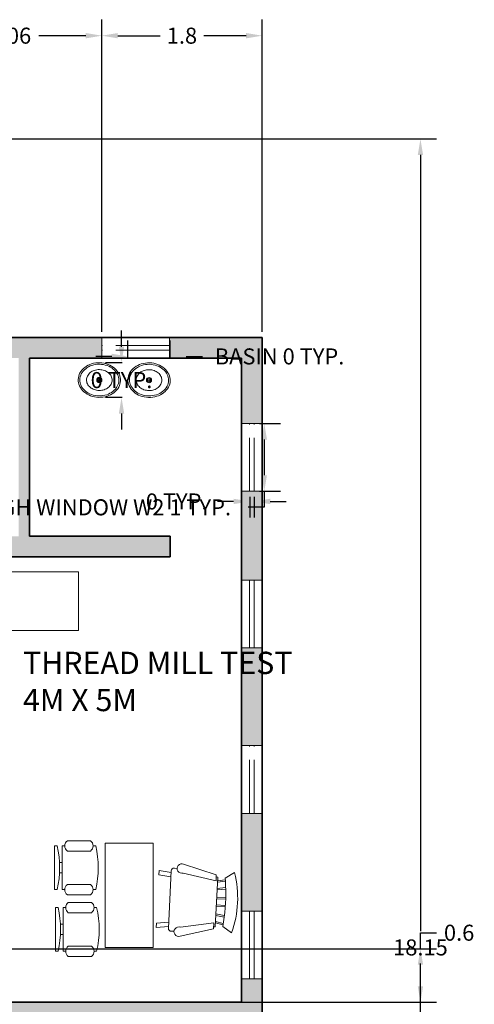
# Model space of a CAD drawing. Units: metres. Extents: x 4298.5 to 4325.2, y 2075 to 2095.8.
# Tile 35 of 35: x 4320.1 to 4325.2, y 2084.8 to 2095.8. Entities that reach past the tile are written whole.
import ezdxf

# ---------------------------------------------------------------- set-up
doc = ezdxf.new("R2010")
doc.units = ezdxf.units.M
doc.linetypes.add('ACAD_ISO02W100', pattern=[15, 12, -3])
for name, color, linetype, lineweight in [('A-ANNO-DIMS', 2, 'Continuous', 18), ('A-AREA-IDEN', 7, 'Continuous', 18), ('A-EQPM', 9, 'Continuous', 18), ('A-FLOR-FIXT', 15, 'Continuous', 18), ('A-FURN', 15, 'Continuous', 18), ('A-GLAZ', 4, 'Continuous', 18), ('A-GLAZ-OVHD', 4, 'ACAD_ISO02W100', 13), ('A-WALL', 7, 'Continuous', 35), ('A-WALL-PATT', 252, 'Continuous', 13)]:
    doc.layers.add(name, color=color, linetype=linetype, lineweight=lineweight)
doc.styles.get("Standard").update_dxf_attribs({"font": 'arial.ttf'})
doc.dimstyles.get("Standard").update_dxf_attribs({"dimtxt": 0.18, "dimasz": 0.18, "dimexe": 0.18, "dimexo": 0.0625, "dimgap": 0.09, "dimtad": 0, "dimtih": 1, "dimtoh": 1, "dimdec": 4, "dimzin": 0, "dimdsep": 46, "dimtxsty": 'Standard', "dimcen": 0.09, "dimadec": 0, "dimazin": 0, "dimtfac": 1, "dimtdec": 4, "dimtofl": 0, "dimtmove": 0, "dimatfit": 3, "dimfxl": 1, "dimtolj": 1, "dimtzin": 0, "dimarcsym": 0})

# ---------------------------------------------------------------- blocks, each defined once
blk = doc.blocks.new('Chair - Desk')
for p, q in [((-8.5, 0), (-8.5, -1)), ((-8.5, 0), (8.5, 0)), ((8.5, 0), (8.5, -1)), ((-8.5, -3), (-8.5, -4)), ((-8.5, -3), (8.5, -3)), ((-2, -3), (-2, -1.9355)), ((2, -1.9576), (2, -3)), ((8.5, -3), (8.5, -4)), ((-10.5, -5), (-10.5, -14)), ((-6.5, -14), (-6.5, -5)), ((6.5, -5), (6.5, -14)), ((10.5, -14), (10.5, -5)), ((-8.5, -15), (-8.5, -16)), ((8.5, -15), (8.5, -16))]:
    blk.add_line(p, q)
for centre, radius, start, end in [((0, 34.625), 36.625, 256.5803, 283.4197), ((-8.5, -6.5), 2.5, 36.8699, 143.1301), ((8.5, -6.5), 2.5, 36.8699, 143.1301), ((-8.5, -12.5), 2.5, 216.8699, 323.1301), ((8.5, -12.5), 2.5, 216.8699, 323.1301), ((0, 19.625), 36.625, 256.5803, 283.4197)]:
    blk.add_arc(centre, radius, start, end)
blk = doc.blocks.new('Chair - Rocking')
for p, q in [((-8, -4.5), (-10, -1.5)), ((8, -4.5), (10, -1.5)), ((-7.5, -4.5), (-7, -7)), ((-6.5, -7), (-7.02225, -4.43)), ((-4.5, -7), (-4.96674, -4.19951)), ((-4, -7), (-4.40532, -4.16272)), ((-1.5, -4.05012), (-1.5, -7)), ((-1, -7), (-1, -4.05012)), ((1, -7), (1, -4.04655)), ((1.5, -4.05012), (1.5, -7)), ((4, -7), (4.40187, -4.18694)), ((4.5, -7), (4.96761, -4.19437)), ((6.5, -7), (7, -4.4057)), ((7.5, -4.5), (7, -7)), ((-9, -7.5), (-12, -18.49999)), ((-7, -7.5), (-9, -7.5)), ((-9, -18.49999), (-7, -7.5)), ((-8.23428, -6.99939), (-8.3093, -7.47958)), ((-8.23041, -7), (8.23915, -7)), ((7, -7.5), (9, -7.5)), ((9, -18.49999), (7, -7.5)), ((8.31071, -7.48854), (8.23449, -7.00073)), ((9, -7.5), (12, -18.49999)), ((-10.36644, -20.64523), (-10.5, -21.49999)), ((-9, -22.49999), (-9.5, -26.49999)), ((0, -22.49999), (-9.5, -22.49999)), ((-8, -26.49999), (-7.5, -22.49999)), ((0, -22.49999), (9.5, -22.49999)), ((8, -26.49999), (7.5, -22.49999)), ((9, -22.49999), (9.5, -26.49999)), ((10.5, -21.49999), (10.3575, -20.58798)), ((-9.5, -26.49999), (-8, -26.49999)), ((9.5, -26.49999), (8, -26.49999))]:
    blk.add_line(p, q)
for centre, radius, start, end in [((0, -34.08333), 34.08333, 72.93847, 107.0615), ((0, -68.25004), 64.25, 93.92211, 97.15267), ((0, -68.25004), 64.25, 82.84733, 93.92211), ((-10.5, -18.99999), 1.58114, 161.5651, 18.43495), ((10.5, -18.99999), 1.58114, 161.5651, 18.43495), ((-9.5, -21.49999), 1, 180, 270), ((9.5, -21.49999), 1, 270, 0)]:
    blk.add_arc(centre, radius, start, end)
blk = doc.blocks.new('Sink - Oval top')
for p, q in [((-1, 0), (1, 0)), ((0, 1), (0, -1))]:
    blk.add_line(p, q)
for points in [[(-12.23, 0.39, 0.117634), (-11.46, -3.36, 0.104469), (-8.88, -6.8, 0.090016), (-5.08, -9.07, 0.08192), (-0.32, -10.02, 0.08192), (4.49, -9.38, 0.090016), (8.42, -7.36, 0.104469), (11.22, -4.09, 0.117634), (12.23, -0.39, 0.117634), (11.46, 3.36, 0.104469), (8.88, 6.8, 0.090016), (5.08, 9.07, 0.08192), (0.32, 10.02, 0.08192), (-4.49, 9.38, 0.090016), (-8.42, 7.36, 0.104469), (-11.22, 4.09, 0.117634)], [(-11.29, 0.16, 0.118622), (-10.52, -3.25, 0.104678), (-8.07, -6.36, 0.089562), (-4.54, -8.37, 0.081185), (-0.13, -9.15, 0.081185), (4.3, -8.49, 0.089562), (7.89, -6.58, 0.104678), (10.42, -3.55, 0.118622), (11.29, -0.16, 0.118622), (10.52, 3.25, 0.104678), (8.07, 6.36, 0.089562), (4.54, 8.37, 0.081185), (0.13, 9.15, 0.081185), (-4.3, 8.49, 0.089562), (-7.89, 6.58, 0.104678), (-10.42, 3.55, 0.118622)], [(-7.42, 0.08, 0.118283), (-6.91, -2.17, 0.104607), (-5.29, -4.21, 0.089718), (-2.97, -5.53, 0.081436), (-0.07, -6.04, 0.081436), (2.84, -5.59, 0.089718), (5.2, -4.33, 0.104607), (6.86, -2.32, 0.118283), (7.42, -0.08, 0.118283), (6.91, 2.17, 0.104607), (5.29, 4.21, 0.089718), (2.97, 5.53, 0.081436), (0.07, 6.04, 0.081436), (-2.84, 5.59, 0.089718), (-5.2, 4.33, 0.104607), (-6.86, 2.32, 0.118283)]]:
    blk.add_lwpolyline(points, format="xyb", close=True)
for radius in [1.5, 1]:
    blk.add_circle((0, 0), radius)
blk = doc.blocks.new('WIN-760-GLASS-HIGH')
at = {"ltscale": 0.05}
for p, q in [((0, 0.76), (0, 0)), ((0.05, 0.76), (0.05, 0))]:
    blk.add_line(p, q, dxfattribs=at)
blk = doc.blocks.new('WIN-760-GLASS')
for p, q in [((0, 0.76), (0, 0)), ((0.05, 0.76), (0.05, 0))]:
    blk.add_line(p, q)
blk = doc.blocks.new('DESK-1175')
blk.add_lwpolyline([(0, 1.173), (0.538, 1.173), (0.538, 0), (0, 0)], close=True)
blk = doc.blocks.new('*D21')
at = {"layer": 'A-ANNO-DIMS', "color": 0, "lineweight": -2, "transparency": 16777216}
for p, q in [((4321.304, 2092.028), (4321.304, 2092.217)), ((4321.78, 2092.028), (4321.78, 2092.217)), ((4321.124, 2092.037), (4320.944, 2092.037)), ((4321.96, 2092.037), (4322.14, 2092.037))]:
    blk.add_line(p, q, dxfattribs=at)
at = {"layer": 'A-ANNO-DIMS', "color": 0, "transparency": 16777216}
for points in [[(4321.124, 2092.067), (4321.124, 2092.007), (4321.304, 2092.037)], [(4321.96, 2092.067), (4321.96, 2092.007), (4321.78, 2092.037)]]:
    blk.add_solid(points, dxfattribs=at)
at = {"layer": 'Defpoints', "color": 0, "transparency": 16777216}
for p in [(4321.304, 2091.966), (4321.78, 2092.037), (4321.78, 2091.966)]:
    blk.add_point(p, dxfattribs=at)
at = {"layer": 'A-ANNO-DIMS', "color": 0, "transparency": 16777216, "insert": (4323.006, 2092.037), "char_height": 0.18, "attachment_point": 5}
blk.add_mtext('\\A1;BASIN 0 TYP.', dxfattribs=at)
blk = doc.blocks.new('*D22')
at = {"layer": 'A-ANNO-DIMS', "color": 0, "lineweight": -2, "transparency": 16777216}
for p, q in [((4321.233, 2092.146), (4321.233, 2092.326)), ((4321.241, 2091.966), (4321.053, 2091.966)), ((4321.241, 2091.576), (4321.053, 2091.576)), ((4321.233, 2091.396), (4321.233, 2091.216))]:
    blk.add_line(p, q, dxfattribs=at)
at = {"layer": 'A-ANNO-DIMS', "color": 0, "transparency": 16777216}
for points in [[(4321.203, 2092.146), (4321.263, 2092.146), (4321.233, 2091.966)], [(4321.203, 2091.396), (4321.263, 2091.396), (4321.233, 2091.576)]]:
    blk.add_solid(points, dxfattribs=at)
at = {"layer": 'Defpoints', "color": 0, "transparency": 16777216}
for p in [(4321.233, 2091.966), (4321.304, 2091.966), (4321.304, 2091.576)]:
    blk.add_point(p, dxfattribs=at)
at = {"layer": 'A-ANNO-DIMS', "color": 0, "transparency": 16777216, "insert": (4321.233, 2091.771), "char_height": 0.18, "attachment_point": 5}
blk.add_mtext('\\A1;0 TYP.', dxfattribs=at)
blk = doc.blocks.new('*D25')
at = {"layer": 'A-ANNO-DIMS', "color": 0, "lineweight": -2, "transparency": 16777216}
for p, q in [((4322.783, 2091.283), (4323.015, 2091.283)), ((4322.835, 2091.103), (4322.835, 2090.703)), ((4322.783, 2090.523), (4323.015, 2090.523)), ((4322.835, 2090.523), (4322.835, 2090.343)), ((4322.835, 2090.343), (4322.655, 2090.343))]:
    blk.add_line(p, q, dxfattribs=at)
at = {"layer": 'A-ANNO-DIMS', "color": 0, "transparency": 16777216}
for points in [[(4322.805, 2091.103), (4322.865, 2091.103), (4322.835, 2091.283)], [(4322.805, 2090.703), (4322.865, 2090.703), (4322.835, 2090.523)]]:
    blk.add_solid(points, dxfattribs=at)
at = {"layer": 'Defpoints', "color": 0, "transparency": 16777216}
for p in [(4322.721, 2091.283), (4322.721, 2090.523), (4322.835, 2090.523)]:
    blk.add_point(p, dxfattribs=at)
at = {"layer": 'A-ANNO-DIMS', "color": 0, "transparency": 16777216, "insert": (4321.042, 2090.343), "char_height": 0.18, "attachment_point": 5}
blk.add_mtext('\\A1;HIGH WINDOW W2 1 TYP.', dxfattribs=at)
blk = doc.blocks.new('*D26')
at = {"layer": 'A-ANNO-DIMS', "color": 0, "lineweight": -2, "transparency": 16777216}
for p, q in [((4322.491, 2090.409), (4322.311, 2090.409)), ((4322.671, 2090.461), (4322.671, 2090.229)), ((4322.721, 2090.461), (4322.721, 2090.229)), ((4322.901, 2090.409), (4323.081, 2090.409))]:
    blk.add_line(p, q, dxfattribs=at)
at = {"layer": 'A-ANNO-DIMS', "color": 0, "transparency": 16777216}
for points in [[(4322.491, 2090.439), (4322.491, 2090.379), (4322.671, 2090.409)], [(4322.901, 2090.439), (4322.901, 2090.379), (4322.721, 2090.409)]]:
    blk.add_solid(points, dxfattribs=at)
at = {"layer": 'Defpoints', "color": 0, "transparency": 16777216}
for p in [(4322.671, 2090.523), (4322.721, 2090.523), (4322.671, 2090.409)]:
    blk.add_point(p, dxfattribs=at)
at = {"layer": 'A-ANNO-DIMS', "color": 0, "transparency": 16777216, "insert": (4321.852, 2090.409), "char_height": 0.18, "attachment_point": 5}
blk.add_mtext('\\A1;0 TYP.', dxfattribs=at)
blk = doc.blocks.new('*D48')
at = {"layer": 'A-ANNO-DIMS', "color": 0, "lineweight": -2, "transparency": 16777216}
for p, q in [((4310.183, 2094.478), (4324.767, 2094.478)), ((4324.587, 2094.298), (4324.587, 2085.585)), ((4324.587, 2076.508), (4324.587, 2085.221)), ((4316.873, 2076.328), (4324.767, 2076.328))]:
    blk.add_line(p, q, dxfattribs=at)
at = {"layer": 'A-ANNO-DIMS', "color": 0, "transparency": 16777216}
for points in [[(4324.557, 2094.298), (4324.617, 2094.298), (4324.587, 2094.478)], [(4324.557, 2076.508), (4324.617, 2076.508), (4324.587, 2076.328)]]:
    blk.add_solid(points, dxfattribs=at)
at = {"layer": 'Defpoints', "color": 0, "transparency": 16777216}
for p in [(4310.121, 2094.478), (4316.811, 2076.328), (4324.587, 2076.328)]:
    blk.add_point(p, dxfattribs=at)
at = {"layer": 'A-ANNO-DIMS', "color": 0, "transparency": 16777216, "insert": (4324.587, 2085.403), "char_height": 0.18, "attachment_point": 5}
blk.add_mtext('\\A1;18.15', dxfattribs=at)
blk = doc.blocks.new('*D58')
at = {"layer": 'A-ANNO-DIMS', "color": 0, "lineweight": -2, "transparency": 16777216}
for p, q in [((4324.587, 2085.388), (4324.587, 2085.568)), ((4324.587, 2085.568), (4324.767, 2085.568)), ((4300.723, 2085.388), (4324.767, 2085.388)), ((4324.587, 2084.968), (4324.587, 2085.208)), ((4300.723, 2084.788), (4324.767, 2084.788))]:
    blk.add_line(p, q, dxfattribs=at)
at = {"layer": 'A-ANNO-DIMS', "color": 0, "transparency": 16777216}
for points in [[(4324.557, 2085.208), (4324.617, 2085.208), (4324.587, 2085.388)], [(4324.557, 2084.968), (4324.617, 2084.968), (4324.587, 2084.788)]]:
    blk.add_solid(points, dxfattribs=at)
at = {"layer": 'Defpoints', "color": 0, "transparency": 16777216}
for p in [(4300.661, 2085.388), (4324.587, 2085.388), (4300.661, 2084.788)]:
    blk.add_point(p, dxfattribs=at)
at = {"layer": 'A-ANNO-DIMS', "color": 0, "transparency": 16777216, "insert": (4325.021, 2085.568), "char_height": 0.18, "attachment_point": 5}
blk.add_mtext('\\A1;0.6', dxfattribs=at)
blk = doc.blocks.new('*D72')
at = {"layer": 'A-ANNO-DIMS', "color": 0, "lineweight": -2, "transparency": 16777216}
for p, q in [((4318.951, 2092.311), (4318.951, 2095.817)), ((4321.011, 2092.311), (4321.011, 2095.817)), ((4319.131, 2095.637), (4319.655, 2095.637)), ((4320.831, 2095.637), (4320.306, 2095.637))]:
    blk.add_line(p, q, dxfattribs=at)
at = {"layer": 'A-ANNO-DIMS', "color": 0, "transparency": 16777216}
for points in [[(4319.131, 2095.667), (4319.131, 2095.607), (4318.951, 2095.637)], [(4320.831, 2095.667), (4320.831, 2095.607), (4321.011, 2095.637)]]:
    blk.add_solid(points, dxfattribs=at)
at = {"layer": 'Defpoints', "color": 0, "transparency": 16777216}
for p in [(4321.011, 2095.637), (4318.951, 2092.248), (4321.011, 2092.248)]:
    blk.add_point(p, dxfattribs=at)
at = {"layer": 'A-ANNO-DIMS', "color": 0, "transparency": 16777216, "insert": (4319.981, 2095.637), "char_height": 0.18, "attachment_point": 5}
blk.add_mtext('\\A1;2.06', dxfattribs=at)
blk = doc.blocks.new('*D73')
at = {"layer": 'A-ANNO-DIMS', "color": 0, "lineweight": -2, "transparency": 16777216}
for p, q in [((4321.011, 2092.311), (4321.011, 2095.817)), ((4322.811, 2092.311), (4322.811, 2095.817)), ((4321.191, 2095.637), (4321.665, 2095.637)), ((4322.631, 2095.637), (4322.156, 2095.637))]:
    blk.add_line(p, q, dxfattribs=at)
at = {"layer": 'A-ANNO-DIMS', "color": 0, "transparency": 16777216}
for points in [[(4321.191, 2095.667), (4321.191, 2095.607), (4321.011, 2095.637)], [(4322.631, 2095.667), (4322.631, 2095.607), (4322.811, 2095.637)]]:
    blk.add_solid(points, dxfattribs=at)
at = {"layer": 'Defpoints', "color": 0, "transparency": 16777216}
for p in [(4322.811, 2095.637), (4321.011, 2092.248), (4322.811, 2092.248)]:
    blk.add_point(p, dxfattribs=at)
at = {"layer": 'A-ANNO-DIMS', "color": 0, "transparency": 16777216, "insert": (4321.911, 2095.637), "char_height": 0.18, "attachment_point": 5}
blk.add_mtext('\\A1;1.8', dxfattribs=at)

msp = doc.modelspace()

# ---------------------------------------------------------------- hatches: boundary and pattern name
at = {"layer": 'A-WALL-PATT'}
h = msp.add_hatch(color=256, dxfattribs=at)
h.dxf.hatch_style = 1
h.paths.add_polyline_path([(4308.7606, 2094.4781), (4308.1606, 2094.4781), (4307.4606, 2094.4781), (4307.4606, 2094.2481), (4308.2706, 2094.2481), (4308.2706, 2094.1281), (4308.3906, 2094.1281), (4308.3906, 2094.2481), (4308.7606, 2094.2481)])
h.paths.add_polyline_path([(4310.1206, 2094.4781), (4309.5206, 2094.4781), (4309.5206, 2094.2481), (4309.8906, 2094.2481), (4309.8906, 2092.2481), (4308.3906, 2092.2481), (4308.3906, 2093.4281), (4308.2706, 2093.4281), (4308.2706, 2092.0181), (4309.8906, 2092.0181), (4309.8906, 2087.0181), (4309.7706, 2087.0181), (4309.7706, 2086.7881), (4309.8906, 2086.7881), (4311.9406, 2086.7881), (4311.9406, 2087.0181), (4310.1206, 2087.0181), (4310.1206, 2089.0181), (4310.2406, 2089.0181), (4310.2406, 2089.1381), (4310.1206, 2089.1381), (4310.1206, 2092.0181), (4310.3078, 2092.0181), (4310.3078, 2092.2481), (4310.1206, 2092.2481)])
h.paths.add_polyline_path([(4311.7406, 2092.2481), (4311.0678, 2092.2481), (4311.0678, 2092.0181), (4311.7406, 2092.0181)], flags=17)
h.paths.add_polyline_path([(4313.1733, 2092.2481), (4312.5006, 2092.2481), (4312.5006, 2092.0181), (4313.1733, 2092.0181)])
h.paths.add_polyline_path([(4314.5378, 2092.2481), (4314.1206, 2092.2481), (4313.9333, 2092.2481), (4313.9333, 2092.0181), (4314.1206, 2092.0181), (4314.1206, 2087.0181), (4314.0006, 2087.0181), (4314.0006, 2086.7881), (4314.1206, 2086.7881), (4315.5718, 2086.7881), (4315.5718, 2087.0181), (4314.3506, 2087.0181), (4314.3506, 2092.0181), (4314.5378, 2092.0181)])
h.paths.add_polyline_path([(4315.9706, 2092.2481), (4315.2978, 2092.2481), (4315.2978, 2092.0181), (4315.9706, 2092.0181)])
h.paths.add_polyline_path([(4317.4033, 2092.2481), (4316.7306, 2092.2481), (4316.7306, 2092.0181), (4317.4033, 2092.0181)])
h.paths.add_polyline_path([(4318.9506, 2092.2481), (4318.3506, 2092.2481), (4318.1633, 2092.2481), (4318.1633, 2092.0181), (4318.3506, 2092.0181), (4318.3506, 2091.8981), (4318.5806, 2091.8981), (4318.5806, 2092.0181), (4318.9506, 2092.0181)])
h.paths.add_polyline_path([(4321.0106, 2092.2481), (4319.7106, 2092.2481), (4319.7106, 2092.0181), (4320.0806, 2092.0181), (4320.0806, 2090.0181), (4318.5806, 2090.0181), (4318.5806, 2091.1981), (4318.3506, 2091.1981), (4318.3506, 2090.0181), (4318.3506, 2087.0181), (4318.2306, 2087.0181), (4318.2306, 2086.7881), (4318.3506, 2086.7881), (4318.3506, 2086.3081), (4318.5806, 2086.3081), (4318.5806, 2089.7881), (4321.7806, 2089.7881), (4321.7806, 2090.0181), (4320.2006, 2090.0181), (4320.2006, 2092.0181), (4321.0106, 2092.0181)])
h.paths.add_polyline_path([(4322.8106, 2092.2481), (4321.7706, 2092.2481), (4321.7706, 2092.0181), (4322.5806, 2092.0181), (4322.5806, 2091.2831), (4322.8106, 2091.2831)])
h.paths.add_polyline_path([(4322.8106, 2090.5231), (4322.5806, 2090.5231), (4322.5806, 2089.7881), (4322.5806, 2089.5254), (4322.8106, 2089.5254), (4322.8106, 2090.0181)])
h.paths.add_polyline_path([(4322.8106, 2088.7654), (4322.5806, 2088.7654), (4322.5806, 2087.6681), (4322.8106, 2087.6681)])
h.paths.add_polyline_path([(4322.8106, 2086.9081), (4322.5806, 2086.9081), (4322.5806, 2085.8107), (4322.8106, 2085.8107)])
h.paths.add_polyline_path([(4322.8106, 2085.0507), (4322.5806, 2085.0507), (4322.5806, 2084.7881), (4318.5806, 2084.7881), (4318.5806, 2085.0581), (4318.5806, 2085.4081), (4318.3506, 2085.4081), (4318.3506, 2084.5581), (4318.3506, 2080.8581), (4318.4706, 2080.8581), (4318.4706, 2082.3281), (4319.2606, 2082.3281), (4319.2606, 2082.5581), (4318.5806, 2082.5581), (4318.5806, 2084.5581), (4320.0806, 2084.5581), (4320.0806, 2083.9381), (4320.3106, 2083.9381), (4320.3106, 2084.5581), (4322.8106, 2084.5581)])
h.paths.add_polyline_path([(4320.3106, 2083.1781), (4320.0806, 2083.1781), (4320.0806, 2082.5581), (4319.9606, 2082.5581), (4319.9606, 2082.3281), (4320.0806, 2082.3281), (4320.0806, 2081.5731), (4320.3106, 2081.5731)], flags=17)
h.paths.add_polyline_path([(4320.3106, 2080.8131), (4320.0806, 2080.8131), (4320.0806, 2080.0581), (4318.4286, 2080.0581), (4318.4286, 2079.8281), (4320.3106, 2079.8281)])
h.paths.add_polyline_path([(4317.3506, 2085.2881), (4316.5718, 2085.2881), (4316.5718, 2085.0581), (4317.3506, 2085.0581)])
h.paths.add_polyline_path([(4315.5718, 2085.2881), (4314.8434, 2085.2881), (4314.8434, 2085.0581), (4315.5718, 2085.0581)])
h.paths.add_polyline_path([(4313.8434, 2085.2881), (4312.9406, 2085.2881), (4312.9406, 2085.0581), (4313.8434, 2085.0581)])
h.paths.add_polyline_path([(4311.9406, 2085.2881), (4311.4406, 2085.2881), (4311.4406, 2085.0581), (4311.9406, 2085.0581)])
h.paths.add_polyline_path([(4317.3306, 2087.0181), (4316.5718, 2087.0181), (4316.5718, 2086.7881), (4317.3306, 2086.7881)])
h.paths.add_polyline_path([(4313.1006, 2089.1381), (4311.1406, 2089.1381), (4311.1406, 2089.0181), (4312.9806, 2089.0181), (4312.9806, 2087.0181), (4312.9406, 2087.0181), (4312.9406, 2086.7881), (4313.1006, 2086.7881), (4313.1006, 2087.0181)])
h.paths.add_polyline_path([(4307.5515, 2087.0181), (4305.8906, 2087.0181), (4305.8906, 2092.2481), (4305.8906, 2094.2481), (4306.7006, 2094.2481), (4306.7006, 2094.4781), (4305.6606, 2094.4781), (4305.6606, 2092.2481), (4305.2906, 2092.2481), (4305.2906, 2092.0181), (4305.6606, 2092.0181), (4305.6606, 2090.0181), (4304.1606, 2090.0181), (4304.1606, 2091.1981), (4304.0406, 2091.1981), (4304.0406, 2089.9081), (4301.5606, 2089.9081), (4301.5606, 2089.7881), (4304.0406, 2089.7881), (4305.6606, 2089.7881), (4305.6606, 2086.6381), (4305.8906, 2086.6381), (4305.8906, 2086.7881), (4307.5515, 2086.7881)])
h.paths.add_polyline_path([(4307.5515, 2085.2881), (4305.8906, 2085.2881), (4305.8906, 2085.4381), (4305.6606, 2085.4381), (4305.6606, 2084.7881), (4305.2906, 2084.7881), (4305.2906, 2084.5581), (4305.6606, 2084.5581), (4305.6606, 2084.02), (4305.8906, 2084.02), (4305.8906, 2084.5581), (4305.8906, 2085.0581), (4307.5515, 2085.0581)])
h.paths.add_polyline_path([(4310.2406, 2085.2881), (4308.5515, 2085.2881), (4308.5515, 2085.0581), (4310.2406, 2085.0581)])
h.paths.add_polyline_path([(4317.4286, 2080.0581), (4316.5718, 2080.0581), (4316.5718, 2079.8281), (4317.4286, 2079.8281)])
h.paths.add_polyline_path([(4315.5718, 2080.0581), (4314.8434, 2080.0581), (4314.8434, 2079.8281), (4315.5718, 2079.8281)])
h.paths.add_polyline_path([(4313.8434, 2080.0581), (4312.9406, 2080.0581), (4312.9406, 2079.8281), (4313.8434, 2079.8281)])
h.paths.add_polyline_path([(4311.9406, 2080.0581), (4311.4406, 2080.0581), (4311.4406, 2079.8281), (4311.9406, 2079.8281)])
h.paths.add_polyline_path([(4310.2406, 2080.0581), (4310.1206, 2080.0581), (4310.1206, 2084.0381), (4309.8906, 2084.0381), (4309.8906, 2080.0581), (4309.1606, 2080.0581), (4309.1606, 2079.8281), (4310.2406, 2079.8281)])
h.paths.add_polyline_path([(4308.1606, 2080.0581), (4307.5106, 2080.0581), (4307.5106, 2080.1781), (4307.3906, 2080.1781), (4307.3906, 2080.0581), (4305.8906, 2080.0581), (4305.8906, 2080.567), (4305.6606, 2080.567), (4305.6606, 2079.8281), (4308.1606, 2079.8281)])
h.paths.add_polyline_path([(4307.5106, 2081.9381), (4309.0906, 2081.9381), (4309.0906, 2082.0581), (4305.8906, 2082.0581), (4305.8906, 2083.26), (4305.6606, 2083.26), (4305.6606, 2081.327), (4305.8906, 2081.327), (4305.8906, 2081.9381), (4307.3906, 2081.9381), (4307.3906, 2080.8781), (4307.5106, 2080.8781)])
h.paths.add_polyline_path([(4304.5306, 2084.7881), (4302.7306, 2084.7881), (4302.7306, 2084.5581), (4304.5306, 2084.5581)])
h.paths.add_polyline_path([(4301.9706, 2084.7881), (4300.6606, 2084.7881), (4300.6606, 2085.0249), (4300.4306, 2085.0249), (4300.4306, 2084.5581), (4301.9706, 2084.5581)])
h.paths.add_polyline_path([(4300.6606, 2086.8843), (4300.4306, 2086.8843), (4300.4306, 2085.7849), (4300.6606, 2085.7849)])
h.paths.add_polyline_path([(4300.6606, 2089.1618), (4300.4306, 2089.1618), (4300.4306, 2087.6443), (4300.6606, 2087.6443)])
h.paths.add_polyline_path([(4300.6606, 2091.0212), (4300.4306, 2091.0212), (4300.4306, 2089.9218), (4300.6606, 2089.9218)])
h.paths.add_polyline_path([(4300.6606, 2092.0181), (4301.9706, 2092.0181), (4301.9706, 2092.2481), (4300.4306, 2092.2481), (4300.4306, 2091.7812), (4300.6606, 2091.7812)])
h.paths.add_polyline_path([(4304.5306, 2092.2481), (4302.7306, 2092.2481), (4302.7306, 2092.0181), (4304.0406, 2092.0181), (4304.0406, 2091.8981), (4304.1606, 2091.8981), (4304.1606, 2092.0181), (4304.5306, 2092.0181)], flags=17)

# ---------------------------------------------------------------- linework, layer by layer
at = {"layer": 'A-EQPM'}
msp.add_lwpolyline([(4319.2513, 2089.6206), (4320.7499, 2089.6206), (4320.7499, 2088.9592), (4319.2513, 2088.9592)], close=True, dxfattribs=at)
at = {"layer": 'A-GLAZ'}
for p, q in [((4321.0106, 2092.0181), (4321.0106, 2092.2481)), ((4321.7706, 2092.0181), (4321.7706, 2092.2481)), ((4322.5806, 2091.2831), (4322.8106, 2091.2831)), ((4322.5806, 2090.5231), (4322.8106, 2090.5231)), ((4322.5806, 2089.5254), (4322.8106, 2089.5254)), ((4322.5806, 2088.7654), (4322.8106, 2088.7654)), ((4322.5806, 2087.6681), (4322.8106, 2087.6681)), ((4322.5806, 2086.9081), (4322.8106, 2086.9081)), ((4322.5806, 2085.8107), (4322.8106, 2085.8107)), ((4322.5806, 2085.0507), (4322.8106, 2085.0507))]:
    msp.add_line(p, q, dxfattribs=at)
at = {"layer": 'A-WALL'}
for p, q in [((4318.3506, 2092.2481), (4322.8106, 2092.2481)), ((4322.8106, 2090.0181), (4322.8106, 2092.2481)), ((4320.2006, 2090.0181), (4320.2006, 2092.0181)), ((4320.2006, 2092.0181), (4322.5806, 2092.0181)), ((4322.5806, 2089.7881), (4322.5806, 2092.0181)), ((4320.2006, 2090.0181), (4321.7806, 2090.0181)), ((4321.7806, 2090.0181), (4321.7806, 2089.7881)), ((4322.8106, 2090.0181), (4322.8106, 2084.5581)), ((4318.5806, 2089.7881), (4321.7806, 2089.7881)), ((4322.5806, 2089.7881), (4322.5806, 2084.7881)), ((4322.5806, 2084.7881), (4318.5806, 2084.7881))]:
    msp.add_line(p, q, dxfattribs=at)

# ---------------------------------------------------------------- block references
at = {"layer": 'A-FLOR-FIXT', "xscale": 0.0193818050953029, "yscale": 0.0193818050953029, "zscale": 0.0193818050953029}
for p in [(4320.9839, 2091.7717), (4321.5418, 2091.7708)]:
    msp.add_blockref('Sink - Oval top', p, dxfattribs=at)
at = {"layer": 'A-FURN'}
for name, p, xscale, yscale, zscale, rotation in [('Chair - Desk', (4320.481, 2086.2974), 0.0288995186862949, 0.0288995186862949, 0.0288995186862949, 89.99999999999999), ('Chair - Rocking', (4322.5351, 2085.9023), 0.0338365474760119, 0.0338365474760119, 0.0338365474760119, 267.1375936308194), ('Chair - Desk', (4320.4917, 2085.6051), 0.0288995186862949, 0.0288995186862949, 0.0288995186862949, 89.99999999999999)]:
    msp.add_blockref(name, p, dxfattribs=dict(at, xscale=xscale, yscale=yscale, zscale=zscale, rotation=rotation))
at = {"layer": 'A-FURN', "rotation": 180}
msp.add_blockref('DESK-1175', (4321.5872, 2086.5737), dxfattribs=at)
at = {"layer": 'A-GLAZ', "rotation": 180}
msp.add_blockref('WIN-760-GLASS', (4322.7206, 2089.5254), dxfattribs=at)
at = {"layer": 'A-GLAZ'}
msp.add_blockref('WIN-760-GLASS', (4322.6706, 2085.0507), dxfattribs=at)
at = {"layer": 'A-GLAZ-OVHD'}
for p, rotation in [((4321.0106, 2092.1581), 269.9999999999317), ((4322.7206, 2091.2831), 180), ((4322.7206, 2087.6681), 180)]:
    msp.add_blockref('WIN-760-GLASS-HIGH', p, dxfattribs=dict(at, rotation=rotation))

# ---------------------------------------------------------------- texts
at = {"layer": 'A-AREA-IDEN', "insert": (4320.1266, 2088.7219), "char_height": 0.25, "attachment_point": 1}
msp.add_mtext_dynamic_manual_height_columns('THREAD MILL TEST \\P4M X 5M', width=3.027226, gutter_width=12.5, heights=[0], dxfattribs=at)

# ---------------------------------------------------------------- dimensions: what is measured, and where the dimension line sits
at = {"layer": 'A-ANNO-DIMS'}
for base, p1, p2, override, picture, middle in [((4321.0106, 2095.6366), (4318.9506, 2092.2481), (4321.0106, 2092.2481), {"dimdec": 2, "dimlfac": 1, "dimrnd": 0, "dimzin": 0, "dimdsep": 46, "dimlunit": 2}, '*D72', (4319.9806, 2095.6366)), ((4322.8106, 2095.6366), (4321.0106, 2092.2481), (4322.8106, 2092.2481), {"dimdec": 1, "dimlfac": 1, "dimrnd": 0, "dimzin": 0, "dimdsep": 46, "dimlunit": 2}, '*D73', (4321.9106, 2095.6366))]:
    dim = msp.add_linear_dim(base=base, p1=p1, p2=p2, dimstyle='Standard', override=override, dxfattribs=at)
    dim.commit()
    dim.dimension.update_dxf_attribs({"geometry": picture, "text_midpoint": middle})
for base, p1, p2, override, picture, middle in [((4324.5871, 2076.3281), (4310.1206, 2094.4781), (4316.8106, 2076.3281), {"dimdec": 2, "dimlfac": 1, "dimrnd": 0, "dimzin": 0, "dimdsep": 46, "dimlunit": 2}, '*D48', (4324.5871, 2085.4031)), ((4324.5871, 2085.3881), (4300.6606, 2084.7881), (4300.6606, 2085.3881), {"dimdec": 1, "dimlfac": 1, "dimrnd": 0, "dimzin": 0, "dimdsep": 46, "dimlunit": 2}, '*D58', (4325.0209, 2085.5681))]:
    dim = msp.add_linear_dim(base=base, p1=p1, p2=p2, angle=90, dimstyle='Standard', override=override, dxfattribs=at)
    dim.commit()
    dim.dimension.update_dxf_attribs({"geometry": picture, "text_midpoint": middle})
dim = msp.add_linear_dim(base=(4321.7797, 2092.0373), p1=(4321.3039, 2091.9659), p2=(4321.7797, 2091.9659), text='BASIN <> TYP.', dimstyle='Standard', override={"dimdec": 0, "dimlfac": 1, "dimrnd": 0, "dimzin": 0, "dimdsep": 46, "dimlunit": 2}, dxfattribs=at)
dim.commit()
dim.dimension.update_dxf_attribs({"geometry": '*D21', "text_midpoint": (4323.0062, 2092.0373)})
for base, p1, p2, angle, text, picture, middle in [((4321.2325, 2091.9659), (4321.3039, 2091.5756), (4321.3039, 2091.9659), 90, '<> TYP.', '*D22', (4321.2325, 2091.7708)), ((4322.8346, 2090.5231), (4322.7206, 2091.2831), (4322.7206, 2090.5231), 270, 'HIGH WINDOW W2 <> TYP.', '*D25', (4321.0419, 2090.3431)), ((4322.6706, 2090.4091), (4322.7206, 2090.5231), (4322.6706, 2090.5231), 180, '<> TYP.', '*D26', (4321.8524, 2090.4091))]:
    dim = msp.add_linear_dim(base=base, p1=p1, p2=p2, angle=angle, text=text, dimstyle='Standard', override={"dimdec": 0, "dimlfac": 1, "dimrnd": 0, "dimzin": 0, "dimdsep": 46, "dimlunit": 2}, dxfattribs=at)
    dim.commit()
    dim.dimension.update_dxf_attribs({"geometry": picture, "text_midpoint": middle})

doc.saveas('drawing.dxf')
